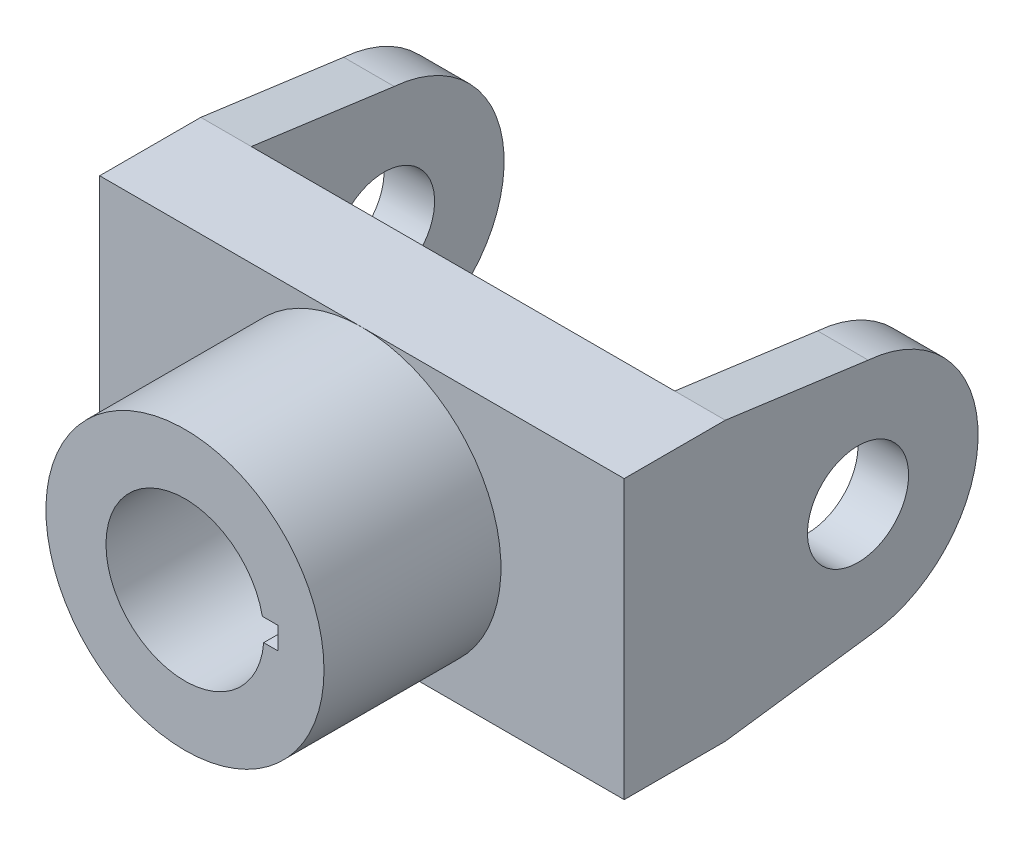
ISO-10303-21;
HEADER;
FILE_DESCRIPTION(('STEP AP214'),'2;1');
FILE_NAME('part.step','',(''),(''),'','','');
FILE_SCHEMA(('AUTOMOTIVE_DESIGN { 1 0 10303 214 1 1 1 1 }'));
ENDSEC;
DATA;
#1=APPLICATION_CONTEXT('core data for automotive mechanical design processes');
#2=APPLICATION_PROTOCOL_DEFINITION('international standard','automotive_design',2000,#1);
#3=PRODUCT_CONTEXT('',#1,'mechanical');
#4=PRODUCT('Part','Part','',(#3));
#5=PRODUCT_RELATED_PRODUCT_CATEGORY('part','',(#4));
#6=PRODUCT_DEFINITION_FORMATION('','',#4);
#7=PRODUCT_DEFINITION_CONTEXT('part definition',#1,'design');
#8=PRODUCT_DEFINITION('design','',#6,#7);
#9=PRODUCT_DEFINITION_SHAPE('','',#8);
#10=(LENGTH_UNIT() NAMED_UNIT(*) SI_UNIT(.MILLI.,.METRE.));
#11=(NAMED_UNIT(*) PLANE_ANGLE_UNIT() SI_UNIT($,.RADIAN.));
#12=(NAMED_UNIT(*) SI_UNIT($,.STERADIAN.) SOLID_ANGLE_UNIT());
#13=UNCERTAINTY_MEASURE_WITH_UNIT(LENGTH_MEASURE(1.E-05),#10,'distance_accuracy_value','');
#14=(GEOMETRIC_REPRESENTATION_CONTEXT(3) GLOBAL_UNCERTAINTY_ASSIGNED_CONTEXT((#13)) GLOBAL_UNIT_ASSIGNED_CONTEXT((#10,
#11,#12)) REPRESENTATION_CONTEXT('',''));
#15=CARTESIAN_POINT('',(0.,0.,0.));
#16=DIRECTION('',(0.,0.,1.));
#17=DIRECTION('',(1.,0.,0.));
#18=AXIS2_PLACEMENT_3D('',#15,#16,#17);
#19=CARTESIAN_POINT('',(0.,0.,0.));
#20=DIRECTION('',(0.,0.,1.));
#21=DIRECTION('',(1.,0.,0.));
#22=AXIS2_PLACEMENT_3D('',#19,#20,#21);
#23=PLANE('',#22);
#24=CARTESIAN_POINT('',(0.,44.,0.));
#25=DIRECTION('',(0.,0.,1.));
#26=DIRECTION('',(1.,0.,0.));
#27=AXIS2_PLACEMENT_3D('',#24,#25,#26);
#28=CIRCLE('',#27,44.);
#29=CARTESIAN_POINT('',(0.,88.,0.));
#30=VERTEX_POINT('',#29);
#31=CARTESIAN_POINT('',(0.,0.,0.));
#32=VERTEX_POINT('',#31);
#33=EDGE_CURVE('E55',#30,#32,#28,.T.);
#34=ORIENTED_EDGE('',*,*,#33,.F.);
#35=DIRECTION('',(-1.,0.,0.));
#36=VECTOR('',#35,1.);
#37=CARTESIAN_POINT('',(83.,88.,0.));
#38=LINE('',#37,#36);
#39=CARTESIAN_POINT('',(-83.,88.,0.));
#40=VERTEX_POINT('',#39);
#41=EDGE_CURVE('E265',#30,#40,#38,.T.);
#42=ORIENTED_EDGE('',*,*,#41,.T.);
#43=DIRECTION('',(0.,-1.,0.));
#44=VECTOR('',#43,1.);
#45=CARTESIAN_POINT('',(-83.,88.,0.));
#46=LINE('',#45,#44);
#47=CARTESIAN_POINT('',(-83.,0.,0.));
#48=VERTEX_POINT('',#47);
#49=EDGE_CURVE('E264',#40,#48,#46,.T.);
#50=ORIENTED_EDGE('',*,*,#49,.T.);
#51=DIRECTION('',(1.,0.,0.));
#52=VECTOR('',#51,1.);
#53=CARTESIAN_POINT('',(0.,0.,0.));
#54=LINE('',#53,#52);
#55=EDGE_CURVE('E258',#48,#32,#54,.T.);
#56=ORIENTED_EDGE('',*,*,#55,.T.);
#57=EDGE_LOOP('',(#34,#42,#50,#56));
#58=FACE_BOUND('',#57,.T.);
#59=ADVANCED_FACE('F41',(#58),#23,.T.);
#60=CARTESIAN_POINT('',(0.,0.,-32.));
#61=DIRECTION('',(0.,0.,1.));
#62=DIRECTION('',(1.,0.,0.));
#63=AXIS2_PLACEMENT_3D('',#60,#61,#62);
#64=PLANE('',#63);
#65=DIRECTION('',(0.,-1.,0.));
#66=VECTOR('',#65,1.);
#67=CARTESIAN_POINT('',(-67.,0.,-32.));
#68=LINE('',#67,#66);
#69=CARTESIAN_POINT('',(-67.,88.,-32.));
#70=VERTEX_POINT('',#69);
#71=CARTESIAN_POINT('',(-67.,0.,-32.));
#72=VERTEX_POINT('',#71);
#73=EDGE_CURVE('E191',#70,#72,#68,.T.);
#74=ORIENTED_EDGE('',*,*,#73,.F.);
#75=DIRECTION('',(-1.,0.,0.));
#76=VECTOR('',#75,1.);
#77=CARTESIAN_POINT('',(83.,88.,-32.));
#78=LINE('',#77,#76);
#79=CARTESIAN_POINT('',(67.,88.,-32.));
#80=VERTEX_POINT('',#79);
#81=EDGE_CURVE('E246',#80,#70,#78,.T.);
#82=ORIENTED_EDGE('',*,*,#81,.F.);
#83=DIRECTION('',(0.,-1.,0.));
#84=VECTOR('',#83,1.);
#85=CARTESIAN_POINT('',(67.,0.,-32.));
#86=LINE('',#85,#84);
#87=CARTESIAN_POINT('',(67.,0.,-32.));
#88=VERTEX_POINT('',#87);
#89=EDGE_CURVE('E218',#80,#88,#86,.T.);
#90=ORIENTED_EDGE('',*,*,#89,.T.);
#91=DIRECTION('',(1.,0.,0.));
#92=VECTOR('',#91,1.);
#93=CARTESIAN_POINT('',(-83.,0.,-32.));
#94=LINE('',#93,#92);
#95=EDGE_CURVE('E253',#72,#88,#94,.T.);
#96=ORIENTED_EDGE('',*,*,#95,.F.);
#97=EDGE_LOOP('',(#74,#82,#90,#96));
#98=FACE_BOUND('',#97,.T.);
#99=ADVANCED_FACE('F309',(#98),#64,.F.);
#100=CARTESIAN_POINT('',(-83.,88.,-32.));
#101=DIRECTION('',(-1.,0.,0.));
#102=DIRECTION('',(0.,0.,1.));
#103=AXIS2_PLACEMENT_3D('',#100,#101,#102);
#104=PLANE('',#103);
#105=CARTESIAN_POINT('',(-83.,44.,-74.));
#106=DIRECTION('',(-1.,0.,0.));
#107=DIRECTION('',(0.,0.,1.));
#108=AXIS2_PLACEMENT_3D('',#105,#106,#107);
#109=CIRCLE('',#108,16.);
#110=CARTESIAN_POINT('',(-83.,44.,-58.));
#111=VERTEX_POINT('',#110);
#112=EDGE_CURVE('E173',#111,#111,#109,.T.);
#113=ORIENTED_EDGE('',*,*,#112,.F.);
#114=EDGE_LOOP('',(#113));
#115=FACE_BOUND('',#114,.T.);
#116=ORIENTED_EDGE('',*,*,#49,.F.);
#117=DIRECTION('',(0.,0.,1.));
#118=VECTOR('',#117,1.);
#119=CARTESIAN_POINT('',(-83.,88.,-32.));
#120=LINE('',#119,#118);
#121=CARTESIAN_POINT('',(-83.,88.,-32.));
#122=VERTEX_POINT('',#121);
#123=EDGE_CURVE('E269',#122,#40,#120,.T.);
#124=ORIENTED_EDGE('',*,*,#123,.F.);
#125=DIRECTION('',(0.,0.134472859534771,0.990917277096601));
#126=VECTOR('',#125,1.);
#127=CARTESIAN_POINT('',(-83.,88.,-32.));
#128=LINE('',#127,#126);
#129=CARTESIAN_POINT('',(-83.,81.8632063807074,-77.221428653868));
#130=VERTEX_POINT('',#129);
#131=EDGE_CURVE('E195',#130,#122,#128,.T.);
#132=ORIENTED_EDGE('',*,*,#131,.F.);
#133=CARTESIAN_POINT('',(-83.,44.,-74.));
#134=DIRECTION('',(1.,0.,0.));
#135=DIRECTION('',(0.,0.,-1.));
#136=AXIS2_PLACEMENT_3D('',#133,#134,#135);
#137=CIRCLE('',#136,38.);
#138=CARTESIAN_POINT('',(-83.,6.19987605648469,-77.8923810007347));
#139=VERTEX_POINT('',#138);
#140=EDGE_CURVE('E210',#139,#130,#137,.T.);
#141=ORIENTED_EDGE('',*,*,#140,.F.);
#142=DIRECTION('',(0.,0.133879786402021,-0.990997579610036));
#143=VECTOR('',#142,1.);
#144=CARTESIAN_POINT('',(-83.,0.,-32.));
#145=LINE('',#144,#143);
#146=CARTESIAN_POINT('',(-83.,0.,-32.));
#147=VERTEX_POINT('',#146);
#148=EDGE_CURVE('E200',#147,#139,#145,.T.);
#149=ORIENTED_EDGE('',*,*,#148,.F.);
#150=DIRECTION('',(0.,0.,1.));
#151=VECTOR('',#150,1.);
#152=CARTESIAN_POINT('',(-83.,0.,-32.));
#153=LINE('',#152,#151);
#154=EDGE_CURVE('E49',#147,#48,#153,.T.);
#155=ORIENTED_EDGE('',*,*,#154,.T.);
#156=EDGE_LOOP('',(#116,#124,#132,#141,#149,#155));
#157=FACE_BOUND('',#156,.T.);
#158=ADVANCED_FACE('F320',(#115,#157),#104,.T.);
#159=CARTESIAN_POINT('',(83.,88.,-32.));
#160=DIRECTION('',(0.,1.,0.));
#161=DIRECTION('',(-1.,0.,0.));
#162=AXIS2_PLACEMENT_3D('',#159,#160,#161);
#163=PLANE('',#162);
#164=CARTESIAN_POINT('',(83.,88.,0.));
#165=VERTEX_POINT('',#164);
#166=EDGE_CURVE('E263',#165,#30,#38,.T.);
#167=ORIENTED_EDGE('',*,*,#166,.F.);
#168=DIRECTION('',(0.,0.,1.));
#169=VECTOR('',#168,1.);
#170=CARTESIAN_POINT('',(83.,88.,-32.));
#171=LINE('',#170,#169);
#172=CARTESIAN_POINT('',(83.,88.,-32.));
#173=VERTEX_POINT('',#172);
#174=EDGE_CURVE('E272',#173,#165,#171,.T.);
#175=ORIENTED_EDGE('',*,*,#174,.F.);
#176=EDGE_CURVE('E252',#173,#80,#78,.T.);
#177=ORIENTED_EDGE('',*,*,#176,.T.);
#178=ORIENTED_EDGE('',*,*,#81,.T.);
#179=DIRECTION('',(-1.,0.,0.));
#180=VECTOR('',#179,1.);
#181=CARTESIAN_POINT('',(-67.,88.,-32.));
#182=LINE('',#181,#180);
#183=EDGE_CURVE('E202',#70,#122,#182,.T.);
#184=ORIENTED_EDGE('',*,*,#183,.T.);
#185=ORIENTED_EDGE('',*,*,#123,.T.);
#186=ORIENTED_EDGE('',*,*,#41,.F.);
#187=EDGE_LOOP('',(#167,#175,#177,#178,#184,#185,#186));
#188=FACE_BOUND('',#187,.T.);
#189=ADVANCED_FACE('F290',(#188),#163,.T.);
#190=CARTESIAN_POINT('',(83.,0.,-32.));
#191=DIRECTION('',(1.,0.,0.));
#192=DIRECTION('',(0.,0.,-1.));
#193=AXIS2_PLACEMENT_3D('',#190,#191,#192);
#194=PLANE('',#193);
#195=CARTESIAN_POINT('',(83.,44.,-74.));
#196=DIRECTION('',(1.,0.,0.));
#197=DIRECTION('',(0.,0.,-1.));
#198=AXIS2_PLACEMENT_3D('',#195,#196,#197);
#199=CIRCLE('',#198,16.);
#200=CARTESIAN_POINT('',(83.,44.,-90.));
#201=VERTEX_POINT('',#200);
#202=EDGE_CURVE('E501',#201,#201,#199,.T.);
#203=ORIENTED_EDGE('',*,*,#202,.F.);
#204=EDGE_LOOP('',(#203));
#205=FACE_BOUND('',#204,.T.);
#206=DIRECTION('',(0.,1.,0.));
#207=VECTOR('',#206,1.);
#208=CARTESIAN_POINT('',(83.,0.,0.));
#209=LINE('',#208,#207);
#210=CARTESIAN_POINT('',(83.,0.,0.));
#211=VERTEX_POINT('',#210);
#212=EDGE_CURVE('E259',#211,#165,#209,.T.);
#213=ORIENTED_EDGE('',*,*,#212,.F.);
#214=DIRECTION('',(0.,0.,1.));
#215=VECTOR('',#214,1.);
#216=CARTESIAN_POINT('',(83.,0.,-32.));
#217=LINE('',#216,#215);
#218=CARTESIAN_POINT('',(83.,0.,-32.));
#219=VERTEX_POINT('',#218);
#220=EDGE_CURVE('E254',#219,#211,#217,.T.);
#221=ORIENTED_EDGE('',*,*,#220,.F.);
#222=DIRECTION('',(0.,0.133879786402021,-0.990997579610036));
#223=VECTOR('',#222,1.);
#224=CARTESIAN_POINT('',(83.,0.,-32.));
#225=LINE('',#224,#223);
#226=CARTESIAN_POINT('',(83.,6.19987605648469,-77.8923810007347));
#227=VERTEX_POINT('',#226);
#228=EDGE_CURVE('E213',#219,#227,#225,.T.);
#229=ORIENTED_EDGE('',*,*,#228,.T.);
#230=CARTESIAN_POINT('',(83.,44.,-74.));
#231=DIRECTION('',(1.,0.,0.));
#232=DIRECTION('',(0.,0.,-1.));
#233=AXIS2_PLACEMENT_3D('',#230,#231,#232);
#234=CIRCLE('',#233,38.);
#235=CARTESIAN_POINT('',(83.,81.8632063807074,-77.221428653868));
#236=VERTEX_POINT('',#235);
#237=EDGE_CURVE('E231',#227,#236,#234,.T.);
#238=ORIENTED_EDGE('',*,*,#237,.T.);
#239=DIRECTION('',(0.,0.134472859534771,0.990917277096601));
#240=VECTOR('',#239,1.);
#241=CARTESIAN_POINT('',(83.,88.,-32.));
#242=LINE('',#241,#240);
#243=EDGE_CURVE('E224',#236,#173,#242,.T.);
#244=ORIENTED_EDGE('',*,*,#243,.T.);
#245=ORIENTED_EDGE('',*,*,#174,.T.);
#246=EDGE_LOOP('',(#213,#221,#229,#238,#244,#245));
#247=FACE_BOUND('',#246,.T.);
#248=ADVANCED_FACE('F278',(#205,#247),#194,.T.);
#249=CARTESIAN_POINT('',(0.,0.,-32.));
#250=DIRECTION('',(0.,-1.,0.));
#251=DIRECTION('',(0.,0.,-1.));
#252=AXIS2_PLACEMENT_3D('',#249,#250,#251);
#253=PLANE('',#252);
#254=ORIENTED_EDGE('',*,*,#55,.F.);
#255=ORIENTED_EDGE('',*,*,#154,.F.);
#256=EDGE_CURVE('E250',#147,#72,#94,.T.);
#257=ORIENTED_EDGE('',*,*,#256,.T.);
#258=ORIENTED_EDGE('',*,*,#95,.T.);
#259=DIRECTION('',(1.,0.,0.));
#260=VECTOR('',#259,1.);
#261=CARTESIAN_POINT('',(67.,0.,-32.));
#262=LINE('',#261,#260);
#263=EDGE_CURVE('E235',#88,#219,#262,.T.);
#264=ORIENTED_EDGE('',*,*,#263,.T.);
#265=ORIENTED_EDGE('',*,*,#220,.T.);
#266=EDGE_CURVE('E244',#32,#211,#54,.T.);
#267=ORIENTED_EDGE('',*,*,#266,.F.);
#268=EDGE_LOOP('',(#254,#255,#257,#258,#264,#265,#267));
#269=FACE_BOUND('',#268,.T.);
#270=ADVANCED_FACE('F43',(#269),#253,.T.);
#271=EDGE_CURVE('E11',#32,#30,#28,.T.);
#272=ORIENTED_EDGE('',*,*,#271,.F.);
#273=ORIENTED_EDGE('',*,*,#266,.T.);
#274=ORIENTED_EDGE('',*,*,#212,.T.);
#275=ORIENTED_EDGE('',*,*,#166,.T.);
#276=EDGE_LOOP('',(#272,#273,#274,#275));
#277=FACE_BOUND('',#276,.T.);
#278=ADVANCED_FACE('F285',(#277),#23,.T.);
#279=CARTESIAN_POINT('',(67.,88.,-32.));
#280=DIRECTION('',(0.,0.990917277096601,-0.134472859534771));
#281=DIRECTION('',(0.,0.134472859534771,0.990917277096601));
#282=AXIS2_PLACEMENT_3D('',#279,#280,#281);
#283=PLANE('',#282);
#284=ORIENTED_EDGE('',*,*,#243,.F.);
#285=DIRECTION('',(1.,0.,0.));
#286=VECTOR('',#285,1.);
#287=CARTESIAN_POINT('',(67.,81.8632063807074,-77.221428653868));
#288=LINE('',#287,#286);
#289=CARTESIAN_POINT('',(67.,81.8632063807074,-77.221428653868));
#290=VERTEX_POINT('',#289);
#291=EDGE_CURVE('E238',#290,#236,#288,.T.);
#292=ORIENTED_EDGE('',*,*,#291,.F.);
#293=DIRECTION('',(0.,0.134472859534771,0.990917277096601));
#294=VECTOR('',#293,1.);
#295=CARTESIAN_POINT('',(67.,88.,-32.));
#296=LINE('',#295,#294);
#297=EDGE_CURVE('E226',#290,#80,#296,.T.);
#298=ORIENTED_EDGE('',*,*,#297,.T.);
#299=ORIENTED_EDGE('',*,*,#176,.F.);
#300=EDGE_LOOP('',(#284,#292,#298,#299));
#301=FACE_BOUND('',#300,.T.);
#302=ADVANCED_FACE('F321',(#301),#283,.T.);
#303=CARTESIAN_POINT('',(67.,44.,-74.));
#304=DIRECTION('',(1.,0.,0.));
#305=DIRECTION('',(0.,0.,-1.));
#306=AXIS2_PLACEMENT_3D('',#303,#304,#305);
#307=CYLINDRICAL_SURFACE('',#306,38.);
#308=ORIENTED_EDGE('',*,*,#237,.F.);
#309=DIRECTION('',(1.,0.,0.));
#310=VECTOR('',#309,1.);
#311=CARTESIAN_POINT('',(67.,6.19987605648469,-77.8923810007347));
#312=LINE('',#311,#310);
#313=CARTESIAN_POINT('',(67.,6.19987605648469,-77.8923810007347));
#314=VERTEX_POINT('',#313);
#315=EDGE_CURVE('E245',#314,#227,#312,.T.);
#316=ORIENTED_EDGE('',*,*,#315,.F.);
#317=CARTESIAN_POINT('',(67.,44.,-74.));
#318=DIRECTION('',(1.,0.,0.));
#319=DIRECTION('',(0.,0.,-1.));
#320=AXIS2_PLACEMENT_3D('',#317,#318,#319);
#321=CIRCLE('',#320,38.);
#322=EDGE_CURVE('E227',#314,#290,#321,.T.);
#323=ORIENTED_EDGE('',*,*,#322,.T.);
#324=ORIENTED_EDGE('',*,*,#291,.T.);
#325=EDGE_LOOP('',(#308,#316,#323,#324));
#326=FACE_BOUND('',#325,.T.);
#327=ADVANCED_FACE('F326',(#326),#307,.T.);
#328=CARTESIAN_POINT('',(67.,0.,-32.));
#329=DIRECTION('',(0.,-0.990997579610036,-0.133879786402021));
#330=DIRECTION('',(0.,0.133879786402021,-0.990997579610036));
#331=AXIS2_PLACEMENT_3D('',#328,#329,#330);
#332=PLANE('',#331);
#333=ORIENTED_EDGE('',*,*,#228,.F.);
#334=ORIENTED_EDGE('',*,*,#263,.F.);
#335=DIRECTION('',(0.,0.133879786402021,-0.990997579610036));
#336=VECTOR('',#335,1.);
#337=CARTESIAN_POINT('',(67.,0.,-32.));
#338=LINE('',#337,#336);
#339=EDGE_CURVE('E225',#88,#314,#338,.T.);
#340=ORIENTED_EDGE('',*,*,#339,.T.);
#341=ORIENTED_EDGE('',*,*,#315,.T.);
#342=EDGE_LOOP('',(#333,#334,#340,#341));
#343=FACE_BOUND('',#342,.T.);
#344=ADVANCED_FACE('F367',(#343),#332,.T.);
#345=CARTESIAN_POINT('',(67.,44.,-74.));
#346=DIRECTION('',(1.,0.,0.));
#347=DIRECTION('',(0.,0.,-1.));
#348=AXIS2_PLACEMENT_3D('',#345,#346,#347);
#349=PLANE('',#348);
#350=CARTESIAN_POINT('',(67.,44.,-74.));
#351=DIRECTION('',(1.,0.,0.));
#352=DIRECTION('',(0.,0.,-1.));
#353=AXIS2_PLACEMENT_3D('',#350,#351,#352);
#354=CIRCLE('',#353,16.);
#355=CARTESIAN_POINT('',(67.,44.,-90.));
#356=VERTEX_POINT('',#355);
#357=EDGE_CURVE('E510',#356,#356,#354,.T.);
#358=ORIENTED_EDGE('',*,*,#357,.T.);
#359=EDGE_LOOP('',(#358));
#360=FACE_BOUND('',#359,.T.);
#361=ORIENTED_EDGE('',*,*,#89,.F.);
#362=ORIENTED_EDGE('',*,*,#297,.F.);
#363=ORIENTED_EDGE('',*,*,#322,.F.);
#364=ORIENTED_EDGE('',*,*,#339,.F.);
#365=EDGE_LOOP('',(#361,#362,#363,#364));
#366=FACE_BOUND('',#365,.T.);
#367=ADVANCED_FACE('F365',(#360,#366),#349,.F.);
#368=CARTESIAN_POINT('',(-67.,0.,-32.));
#369=DIRECTION('',(0.,0.990997579610036,0.133879786402021));
#370=DIRECTION('',(0.,-0.133879786402021,0.990997579610036));
#371=AXIS2_PLACEMENT_3D('',#368,#369,#370);
#372=PLANE('',#371);
#373=ORIENTED_EDGE('',*,*,#148,.T.);
#374=DIRECTION('',(-1.,0.,0.));
#375=VECTOR('',#374,1.);
#376=CARTESIAN_POINT('',(-67.,6.19987605648469,-77.8923810007347));
#377=LINE('',#376,#375);
#378=CARTESIAN_POINT('',(-67.,6.19987605648469,-77.8923810007347));
#379=VERTEX_POINT('',#378);
#380=EDGE_CURVE('E209',#379,#139,#377,.T.);
#381=ORIENTED_EDGE('',*,*,#380,.F.);
#382=DIRECTION('',(0.,0.133879786402021,-0.990997579610036));
#383=VECTOR('',#382,1.);
#384=CARTESIAN_POINT('',(-67.,0.,-32.));
#385=LINE('',#384,#383);
#386=EDGE_CURVE('E201',#72,#379,#385,.T.);
#387=ORIENTED_EDGE('',*,*,#386,.F.);
#388=ORIENTED_EDGE('',*,*,#256,.F.);
#389=EDGE_LOOP('',(#373,#381,#387,#388));
#390=FACE_BOUND('',#389,.T.);
#391=ADVANCED_FACE('F355',(#390),#372,.F.);
#392=CARTESIAN_POINT('',(-67.,44.,-74.));
#393=DIRECTION('',(-1.,0.,0.));
#394=DIRECTION('',(0.,0.,1.));
#395=AXIS2_PLACEMENT_3D('',#392,#393,#394);
#396=CYLINDRICAL_SURFACE('',#395,38.);
#397=ORIENTED_EDGE('',*,*,#140,.T.);
#398=DIRECTION('',(-1.,0.,0.));
#399=VECTOR('',#398,1.);
#400=CARTESIAN_POINT('',(-67.,81.8632063807074,-77.221428653868));
#401=LINE('',#400,#399);
#402=CARTESIAN_POINT('',(-67.,81.8632063807074,-77.221428653868));
#403=VERTEX_POINT('',#402);
#404=EDGE_CURVE('E212',#403,#130,#401,.T.);
#405=ORIENTED_EDGE('',*,*,#404,.F.);
#406=CARTESIAN_POINT('',(-67.,44.,-74.));
#407=DIRECTION('',(1.,0.,0.));
#408=DIRECTION('',(0.,0.,-1.));
#409=AXIS2_PLACEMENT_3D('',#406,#407,#408);
#410=CIRCLE('',#409,38.);
#411=EDGE_CURVE('E203',#379,#403,#410,.T.);
#412=ORIENTED_EDGE('',*,*,#411,.F.);
#413=ORIENTED_EDGE('',*,*,#380,.T.);
#414=EDGE_LOOP('',(#397,#405,#412,#413));
#415=FACE_BOUND('',#414,.T.);
#416=ADVANCED_FACE('F372',(#415),#396,.T.);
#417=CARTESIAN_POINT('',(-67.,88.,-32.));
#418=DIRECTION('',(0.,-0.990917277096601,0.134472859534771));
#419=DIRECTION('',(0.,-0.134472859534771,-0.990917277096601));
#420=AXIS2_PLACEMENT_3D('',#417,#418,#419);
#421=PLANE('',#420);
#422=ORIENTED_EDGE('',*,*,#131,.T.);
#423=ORIENTED_EDGE('',*,*,#183,.F.);
#424=DIRECTION('',(0.,0.134472859534771,0.990917277096601));
#425=VECTOR('',#424,1.);
#426=CARTESIAN_POINT('',(-67.,88.,-32.));
#427=LINE('',#426,#425);
#428=EDGE_CURVE('E196',#403,#70,#427,.T.);
#429=ORIENTED_EDGE('',*,*,#428,.F.);
#430=ORIENTED_EDGE('',*,*,#404,.T.);
#431=EDGE_LOOP('',(#422,#423,#429,#430));
#432=FACE_BOUND('',#431,.T.);
#433=ADVANCED_FACE('F301',(#432),#421,.F.);
#434=CARTESIAN_POINT('',(-67.,44.,-74.));
#435=DIRECTION('',(-1.,0.,0.));
#436=DIRECTION('',(0.,0.,-1.));
#437=AXIS2_PLACEMENT_3D('',#434,#435,#436);
#438=PLANE('',#437);
#439=CARTESIAN_POINT('',(-67.,44.,-74.));
#440=DIRECTION('',(-1.,0.,0.));
#441=DIRECTION('',(0.,0.,1.));
#442=AXIS2_PLACEMENT_3D('',#439,#440,#441);
#443=CIRCLE('',#442,16.);
#444=CARTESIAN_POINT('',(-67.,44.,-58.));
#445=VERTEX_POINT('',#444);
#446=EDGE_CURVE('E44',#445,#445,#443,.T.);
#447=ORIENTED_EDGE('',*,*,#446,.T.);
#448=EDGE_LOOP('',(#447));
#449=FACE_BOUND('',#448,.T.);
#450=ORIENTED_EDGE('',*,*,#73,.T.);
#451=ORIENTED_EDGE('',*,*,#386,.T.);
#452=ORIENTED_EDGE('',*,*,#411,.T.);
#453=ORIENTED_EDGE('',*,*,#428,.T.);
#454=EDGE_LOOP('',(#450,#451,#452,#453));
#455=FACE_BOUND('',#454,.T.);
#456=ADVANCED_FACE('F293',(#449,#455),#438,.F.);
#457=CARTESIAN_POINT('',(0.,44.,56.));
#458=DIRECTION('',(0.,0.,-1.));
#459=DIRECTION('',(-1.,0.,0.));
#460=AXIS2_PLACEMENT_3D('',#457,#458,#459);
#461=CYLINDRICAL_SURFACE('',#460,44.);
#462=CARTESIAN_POINT('',(0.,44.,56.));
#463=DIRECTION('',(0.,0.,1.));
#464=DIRECTION('',(1.,0.,0.));
#465=AXIS2_PLACEMENT_3D('',#462,#463,#464);
#466=CIRCLE('',#465,44.);
#467=CARTESIAN_POINT('',(44.,44.,56.));
#468=VERTEX_POINT('',#467);
#469=EDGE_CURVE('E188',#468,#468,#466,.T.);
#470=ORIENTED_EDGE('',*,*,#469,.F.);
#471=EDGE_LOOP('',(#470));
#472=FACE_BOUND('',#471,.T.);
#473=ORIENTED_EDGE('',*,*,#33,.T.);
#474=ORIENTED_EDGE('',*,*,#271,.T.);
#475=EDGE_LOOP('',(#473,#474));
#476=FACE_BOUND('',#475,.T.);
#477=ADVANCED_FACE('F295',(#472,#476),#461,.T.);
#478=CARTESIAN_POINT('',(0.,44.,56.));
#479=DIRECTION('',(0.,0.,1.));
#480=DIRECTION('',(1.,0.,0.));
#481=AXIS2_PLACEMENT_3D('',#478,#479,#480);
#482=PLANE('',#481);
#483=CARTESIAN_POINT('',(0.,44.,56.));
#484=DIRECTION('',(0.,0.,1.));
#485=DIRECTION('',(1.,0.,0.));
#486=AXIS2_PLACEMENT_3D('',#483,#484,#485);
#487=CIRCLE('',#486,25.);
#488=CARTESIAN_POINT('',(24.4948974278318,49.,56.));
#489=VERTEX_POINT('',#488);
#490=CARTESIAN_POINT('',(24.9198715887542,42.,56.));
#491=VERTEX_POINT('',#490);
#492=EDGE_CURVE('E56',#489,#491,#487,.T.);
#493=ORIENTED_EDGE('',*,*,#492,.F.);
#494=DIRECTION('',(-1.,0.,0.));
#495=VECTOR('',#494,1.);
#496=CARTESIAN_POINT('',(24.4948974278318,49.,56.));
#497=LINE('',#496,#495);
#498=CARTESIAN_POINT('',(29.4948974278318,49.,56.));
#499=VERTEX_POINT('',#498);
#500=EDGE_CURVE('E166',#499,#489,#497,.T.);
#501=ORIENTED_EDGE('',*,*,#500,.F.);
#502=DIRECTION('',(0.,1.,0.));
#503=VECTOR('',#502,1.);
#504=CARTESIAN_POINT('',(29.4948974278318,49.,56.));
#505=LINE('',#504,#503);
#506=CARTESIAN_POINT('',(29.4948974278318,42.,56.));
#507=VERTEX_POINT('',#506);
#508=EDGE_CURVE('E174',#507,#499,#505,.T.);
#509=ORIENTED_EDGE('',*,*,#508,.F.);
#510=DIRECTION('',(1.,0.,0.));
#511=VECTOR('',#510,1.);
#512=CARTESIAN_POINT('',(29.4948974278318,42.,56.));
#513=LINE('',#512,#511);
#514=EDGE_CURVE('E182',#491,#507,#513,.T.);
#515=ORIENTED_EDGE('',*,*,#514,.F.);
#516=EDGE_LOOP('',(#493,#501,#509,#515));
#517=FACE_BOUND('',#516,.T.);
#518=ORIENTED_EDGE('',*,*,#469,.T.);
#519=EDGE_LOOP('',(#518));
#520=FACE_BOUND('',#519,.T.);
#521=ADVANCED_FACE('F294',(#517,#520),#482,.T.);
#522=CARTESIAN_POINT('',(0.,44.,0.));
#523=DIRECTION('',(0.,0.,1.));
#524=DIRECTION('',(1.,0.,0.));
#525=AXIS2_PLACEMENT_3D('',#522,#523,#524);
#526=CYLINDRICAL_SURFACE('',#525,25.);
#527=ORIENTED_EDGE('',*,*,#492,.T.);
#528=DIRECTION('',(0.,0.,1.));
#529=VECTOR('',#528,1.);
#530=CARTESIAN_POINT('',(24.9198715887542,42.,0.));
#531=LINE('',#530,#529);
#532=CARTESIAN_POINT('',(24.9198715887542,42.,0.));
#533=VERTEX_POINT('',#532);
#534=EDGE_CURVE('E150',#533,#491,#531,.T.);
#535=ORIENTED_EDGE('',*,*,#534,.F.);
#536=CARTESIAN_POINT('',(0.,44.,0.));
#537=DIRECTION('',(0.,0.,1.));
#538=DIRECTION('',(1.,0.,0.));
#539=AXIS2_PLACEMENT_3D('',#536,#537,#538);
#540=CIRCLE('',#539,25.);
#541=CARTESIAN_POINT('',(24.4948974278318,49.,0.));
#542=VERTEX_POINT('',#541);
#543=EDGE_CURVE('E151',#542,#533,#540,.T.);
#544=ORIENTED_EDGE('',*,*,#543,.F.);
#545=DIRECTION('',(0.,0.,1.));
#546=VECTOR('',#545,1.);
#547=CARTESIAN_POINT('',(24.4948974278318,49.,0.));
#548=LINE('',#547,#546);
#549=EDGE_CURVE('E183',#542,#489,#548,.T.);
#550=ORIENTED_EDGE('',*,*,#549,.T.);
#551=EDGE_LOOP('',(#527,#535,#544,#550));
#552=FACE_BOUND('',#551,.T.);
#553=ADVANCED_FACE('F149',(#552),#526,.F.);
#554=CARTESIAN_POINT('',(24.4948974278318,49.,0.));
#555=DIRECTION('',(0.,1.,0.));
#556=DIRECTION('',(0.,0.,1.));
#557=AXIS2_PLACEMENT_3D('',#554,#555,#556);
#558=PLANE('',#557);
#559=ORIENTED_EDGE('',*,*,#500,.T.);
#560=ORIENTED_EDGE('',*,*,#549,.F.);
#561=DIRECTION('',(-1.,0.,0.));
#562=VECTOR('',#561,1.);
#563=CARTESIAN_POINT('',(24.4948974278318,49.,0.));
#564=LINE('',#563,#562);
#565=CARTESIAN_POINT('',(29.4948974278318,49.,0.));
#566=VERTEX_POINT('',#565);
#567=EDGE_CURVE('E160',#566,#542,#564,.T.);
#568=ORIENTED_EDGE('',*,*,#567,.F.);
#569=DIRECTION('',(0.,0.,1.));
#570=VECTOR('',#569,1.);
#571=CARTESIAN_POINT('',(29.4948974278318,49.,0.));
#572=LINE('',#571,#570);
#573=EDGE_CURVE('E189',#566,#499,#572,.T.);
#574=ORIENTED_EDGE('',*,*,#573,.T.);
#575=EDGE_LOOP('',(#559,#560,#568,#574));
#576=FACE_BOUND('',#575,.T.);
#577=ADVANCED_FACE('F449',(#576),#558,.F.);
#578=CARTESIAN_POINT('',(29.4948974278318,49.,0.));
#579=DIRECTION('',(1.,0.,0.));
#580=DIRECTION('',(0.,0.,-1.));
#581=AXIS2_PLACEMENT_3D('',#578,#579,#580);
#582=PLANE('',#581);
#583=ORIENTED_EDGE('',*,*,#508,.T.);
#584=ORIENTED_EDGE('',*,*,#573,.F.);
#585=DIRECTION('',(0.,1.,0.));
#586=VECTOR('',#585,1.);
#587=CARTESIAN_POINT('',(29.4948974278318,49.,0.));
#588=LINE('',#587,#586);
#589=CARTESIAN_POINT('',(29.4948974278318,42.,0.));
#590=VERTEX_POINT('',#589);
#591=EDGE_CURVE('E164',#590,#566,#588,.T.);
#592=ORIENTED_EDGE('',*,*,#591,.F.);
#593=DIRECTION('',(0.,0.,1.));
#594=VECTOR('',#593,1.);
#595=CARTESIAN_POINT('',(29.4948974278318,42.,0.));
#596=LINE('',#595,#594);
#597=EDGE_CURVE('E156',#590,#507,#596,.T.);
#598=ORIENTED_EDGE('',*,*,#597,.T.);
#599=EDGE_LOOP('',(#583,#584,#592,#598));
#600=FACE_BOUND('',#599,.T.);
#601=ADVANCED_FACE('F457',(#600),#582,.F.);
#602=CARTESIAN_POINT('',(29.4948974278318,42.,0.));
#603=DIRECTION('',(0.,-1.,0.));
#604=DIRECTION('',(1.,0.,0.));
#605=AXIS2_PLACEMENT_3D('',#602,#603,#604);
#606=PLANE('',#605);
#607=ORIENTED_EDGE('',*,*,#514,.T.);
#608=ORIENTED_EDGE('',*,*,#597,.F.);
#609=DIRECTION('',(1.,0.,0.));
#610=VECTOR('',#609,1.);
#611=CARTESIAN_POINT('',(29.4948974278318,42.,0.));
#612=LINE('',#611,#610);
#613=EDGE_CURVE('E159',#533,#590,#612,.T.);
#614=ORIENTED_EDGE('',*,*,#613,.F.);
#615=ORIENTED_EDGE('',*,*,#534,.T.);
#616=EDGE_LOOP('',(#607,#608,#614,#615));
#617=FACE_BOUND('',#616,.T.);
#618=ADVANCED_FACE('F161',(#617),#606,.F.);
#619=CARTESIAN_POINT('',(0.,44.,0.));
#620=DIRECTION('',(0.,0.,1.));
#621=DIRECTION('',(1.,0.,0.));
#622=AXIS2_PLACEMENT_3D('',#619,#620,#621);
#623=PLANE('',#622);
#624=ORIENTED_EDGE('',*,*,#543,.T.);
#625=ORIENTED_EDGE('',*,*,#613,.T.);
#626=ORIENTED_EDGE('',*,*,#591,.T.);
#627=ORIENTED_EDGE('',*,*,#567,.T.);
#628=EDGE_LOOP('',(#624,#625,#626,#627));
#629=FACE_BOUND('',#628,.T.);
#630=ADVANCED_FACE('F170',(#629),#623,.T.);
#631=CARTESIAN_POINT('',(-172.,44.,-74.));
#632=DIRECTION('',(1.,0.,0.));
#633=DIRECTION('',(0.,0.,-1.));
#634=AXIS2_PLACEMENT_3D('',#631,#632,#633);
#635=CYLINDRICAL_SURFACE('',#634,16.);
#636=ORIENTED_EDGE('',*,*,#112,.T.);
#637=EDGE_LOOP('',(#636));
#638=FACE_BOUND('',#637,.T.);
#639=ORIENTED_EDGE('',*,*,#446,.F.);
#640=EDGE_LOOP('',(#639));
#641=FACE_BOUND('',#640,.T.);
#642=ADVANCED_FACE('F485',(#638,#641),#635,.F.);
#643=ORIENTED_EDGE('',*,*,#202,.T.);
#644=EDGE_LOOP('',(#643));
#645=FACE_BOUND('',#644,.T.);
#646=ORIENTED_EDGE('',*,*,#357,.F.);
#647=EDGE_LOOP('',(#646));
#648=FACE_BOUND('',#647,.T.);
#649=ADVANCED_FACE('F489',(#645,#648),#635,.F.);
#650=CLOSED_SHELL('',(#59,#99,#158,#189,#248,#270,#278,#302,#327,#344,#367,#391,#416,#433,#456,
#477,#521,#553,#577,#601,#618,#630,#642,#649));
#651=MANIFOLD_SOLID_BREP('B2',#650);
#652=ADVANCED_BREP_SHAPE_REPRESENTATION('',(#18,#651),#14);
#653=SHAPE_DEFINITION_REPRESENTATION(#9,#652);
ENDSEC;
END-ISO-10303-21;
